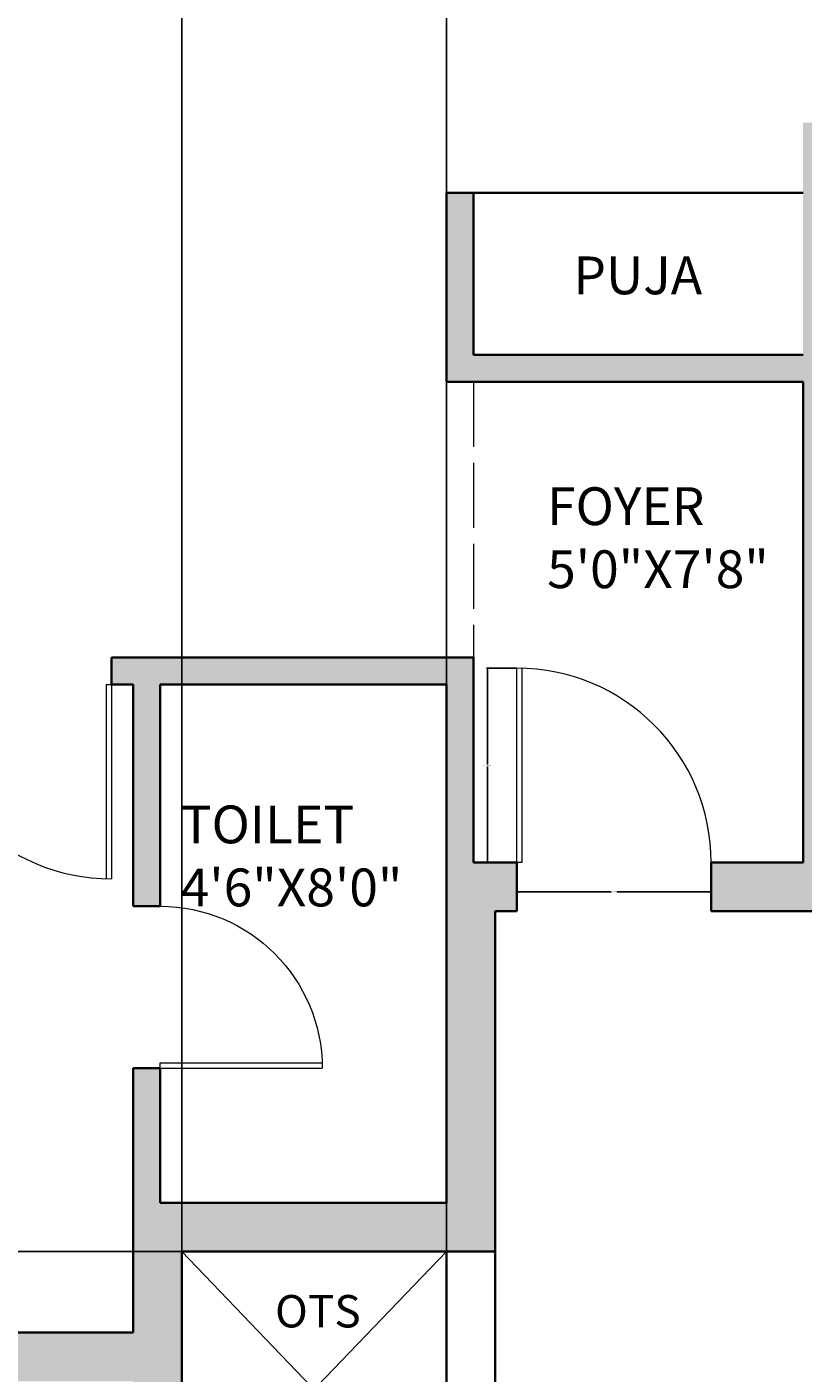
# Model space of a CAD drawing. Units: inches. Extents: x 2540 to 3167, y 3083 to 4007.
# Tile 11 of 15: x 2782 to 2926, y 3542 to 3791. Entities that reach past the tile are written whole.
import ezdxf

# ---------------------------------------------------------------- set-up
doc = ezdxf.new("R2010")
doc.units = ezdxf.units.IN
doc.linetypes.add('ACAD_ISO02W100', pattern=[15, 12, -3])
for name, color, linetype, lineweight in [('A-ANNO-DIMS', 2, 'Continuous', 18), ('A-AREA-IDEN', 7, 'Continuous', 18), ('A-DOOR', 4, 'Continuous', 18), ('A-FLOR-OPEN', 8, 'Continuous', 13)]:
    doc.layers.add(name, color=color, linetype=linetype, lineweight=lineweight)
for name, color, linetype, lineweight, true_color in [('A-WALL', 143, 'Continuous', 35, 0x7aafdf), ('A-WALL-OVHD', 143, 'ACAD_ISO02W100', 18, 0x7aafdf), ('A-WALL-PATT', 143, 'Continuous', 13, 0x7aafdf)]:
    doc.layers.add(name, color=color, linetype=linetype, lineweight=lineweight, true_color=true_color)
doc.styles.get("Standard").update_dxf_attribs({"font": 'arial.ttf'})
doc.dimstyles.get("Standard").update_dxf_attribs({"dimtxt": 0.18, "dimasz": 0.18, "dimexe": 0.18, "dimexo": 0.0625, "dimgap": 0.09, "dimtad": 0, "dimtih": 1, "dimtoh": 1, "dimdec": 4, "dimzin": 0, "dimdsep": 46, "dimtxsty": 'Standard', "dimcen": 0.09, "dimadec": 0, "dimazin": 0, "dimtfac": 1, "dimtdec": 4, "dimtofl": 0, "dimtmove": 0, "dimatfit": 3, "dimfxl": 1, "dimtolj": 1, "dimtzin": 0, "dimarcsym": 0})

# ---------------------------------------------------------------- blocks, each defined once
blk = doc.blocks.new('DOOR-SWING-36IN')
for p, q in [((36, 0), (0, 0)), ((36, 1), (0.01, 1)), ((36, 1), (36, 0))]:
    blk.add_line(p, q)
blk.add_arc((36, 0), 36, 90, 180)
blk = doc.blocks.new('DOOR-SWING-30IN')
for p, q in [((0, 0), (0, 30)), ((1, 0), (1, 29.98)), ((0, 0), (1, 0))]:
    blk.add_line(p, q)
blk.add_arc((0, 0), 30, 0, 90)
blk = doc.blocks.new('*D19')
at = {"layer": 'A-ANNO-DIMS', "color": 0, "lineweight": -2, "transparency": 16777216}
for p, q in [((2872.45, 3672.71), (2866.93, 3672.71)), ((2867.11, 3672.53), (2867.11, 3654.9)), ((2867.11, 3636.89), (2867.11, 3654.53)), ((2872.45, 3636.71), (2866.93, 3636.71))]:
    blk.add_line(p, q, dxfattribs=at)
at = {"layer": 'A-ANNO-DIMS', "color": 0, "transparency": 16777216}
for points in [[(2867.08, 3672.53), (2867.14, 3672.53), (2867.11, 3672.71)], [(2867.08, 3636.89), (2867.14, 3636.89), (2867.11, 3636.71)]]:
    blk.add_solid(points, dxfattribs=at)
at = {"layer": 'Defpoints', "color": 0, "transparency": 16777216}
for p in [(2872.51, 3672.71), (2867.11, 3636.71), (2872.51, 3636.71)]:
    blk.add_point(p, dxfattribs=at)
at = {"layer": 'A-ANNO-DIMS', "color": 0, "transparency": 16777216, "insert": (2867.11, 3654.71), "char_height": 0.18, "attachment_point": 5}
blk.add_mtext('\\A1;DOOR 36 TYP.', dxfattribs=at)
blk = doc.blocks.new('*D20')
at = {"layer": 'A-ANNO-DIMS', "color": 0, "lineweight": -2, "transparency": 16777216}
for p, q in [((2872.51, 3636.65), (2872.51, 3631.13)), ((2908.51, 3636.65), (2908.51, 3631.13)), ((2872.69, 3631.31), (2889.98, 3631.31)), ((2908.33, 3631.31), (2891.04, 3631.31))]:
    blk.add_line(p, q, dxfattribs=at)
at = {"layer": 'A-ANNO-DIMS', "color": 0, "transparency": 16777216}
for points in [[(2872.69, 3631.34), (2872.69, 3631.28), (2872.51, 3631.31)], [(2908.33, 3631.34), (2908.33, 3631.28), (2908.51, 3631.31)]]:
    blk.add_solid(points, dxfattribs=at)
at = {"layer": 'Defpoints', "color": 0, "transparency": 16777216}
for p in [(2872.51, 3636.71), (2908.51, 3636.71), (2908.51, 3631.31)]:
    blk.add_point(p, dxfattribs=at)
at = {"layer": 'A-ANNO-DIMS', "color": 0, "transparency": 16777216, "insert": (2890.51, 3631.31), "char_height": 0.18, "attachment_point": 5}
blk.add_mtext('\\A1;36 TYP.', dxfattribs=at)
blk = doc.blocks.new('*D44')
at = {"layer": 'A-ANNO-DIMS', "color": 0, "lineweight": -2, "transparency": 16777216}
for p, q in [((2771.45, 3964.71), (2540.23, 3964.71)), ((2540.41, 3964.53), (2540.41, 3545.4)), ((2540.41, 3125.89), (2540.41, 3545.03)), ((2810.45, 3125.71), (2540.23, 3125.71))]:
    blk.add_line(p, q, dxfattribs=at)
at = {"layer": 'A-ANNO-DIMS', "color": 0, "transparency": 16777216}
for points in [[(2540.38, 3964.53), (2540.44, 3964.53), (2540.41, 3964.71)], [(2540.38, 3125.89), (2540.44, 3125.89), (2540.41, 3125.71)]]:
    blk.add_solid(points, dxfattribs=at)
at = {"layer": 'Defpoints', "color": 0, "transparency": 16777216}
for p in [(2540.41, 3964.71), (2771.51, 3964.71), (2810.51, 3125.71)]:
    blk.add_point(p, dxfattribs=at)
at = {"layer": 'A-ANNO-DIMS', "color": 0, "transparency": 16777216, "insert": (2540.41, 3545.21), "char_height": 0.18, "attachment_point": 5}
blk.add_mtext('\\A1;839', dxfattribs=at)
blk = doc.blocks.new('*D55')
at = {"layer": 'A-ANNO-DIMS', "color": 0, "lineweight": -2, "transparency": 16777216}
for p, q in [((2868.51, 3564.65), (2868.51, 3083.43)), ((2930.51, 3543.65), (2930.51, 3083.43)), ((2868.69, 3083.61), (2899.29, 3083.61)), ((2930.33, 3083.61), (2899.73, 3083.61))]:
    blk.add_line(p, q, dxfattribs=at)
at = {"layer": 'A-ANNO-DIMS', "color": 0, "transparency": 16777216}
for points in [[(2868.69, 3083.64), (2868.69, 3083.58), (2868.51, 3083.61)], [(2930.33, 3083.64), (2930.33, 3083.58), (2930.51, 3083.61)]]:
    blk.add_solid(points, dxfattribs=at)
at = {"layer": 'Defpoints', "color": 0, "transparency": 16777216}
for p in [(2868.51, 3564.71), (2930.51, 3543.71), (2930.51, 3083.61)]:
    blk.add_point(p, dxfattribs=at)
at = {"layer": 'A-ANNO-DIMS', "color": 0, "transparency": 16777216, "insert": (2899.51, 3083.61), "char_height": 0.18, "attachment_point": 5}
blk.add_mtext('\\A1;62', dxfattribs=at)
blk = doc.blocks.new('*D56')
at = {"layer": 'A-ANNO-DIMS', "color": 0, "lineweight": -2, "transparency": 16777216}
for p, q in [((2810.51, 3564.78), (2810.51, 4006.99)), ((2810.69, 4006.81), (2834.79, 4006.81)), ((2859.33, 4006.81), (2835.23, 4006.81)), ((2859.51, 3564.78), (2859.51, 4006.99))]:
    blk.add_line(p, q, dxfattribs=at)
at = {"layer": 'A-ANNO-DIMS', "color": 0, "transparency": 16777216}
for points in [[(2810.69, 4006.84), (2810.69, 4006.78), (2810.51, 4006.81)], [(2859.33, 4006.84), (2859.33, 4006.78), (2859.51, 4006.81)]]:
    blk.add_solid(points, dxfattribs=at)
at = {"layer": 'Defpoints', "color": 0, "transparency": 16777216}
for p in [(2859.51, 4006.81), (2810.51, 3564.71), (2859.51, 3564.71)]:
    blk.add_point(p, dxfattribs=at)
at = {"layer": 'A-ANNO-DIMS', "color": 0, "transparency": 16777216, "insert": (2835.01, 4006.81), "char_height": 0.18, "attachment_point": 5}
blk.add_mtext('\\A1;49', dxfattribs=at)
blk = doc.blocks.new('*D57')
at = {"layer": 'A-ANNO-DIMS', "color": 0, "lineweight": -2, "transparency": 16777216}
for p, q in [((2810.45, 3564.71), (2540.23, 3564.71)), ((2540.41, 3564.53), (2540.41, 3539.4)), ((2540.41, 3513.89), (2540.41, 3539.03)), ((2810.45, 3513.71), (2540.23, 3513.71))]:
    blk.add_line(p, q, dxfattribs=at)
at = {"layer": 'A-ANNO-DIMS', "color": 0, "transparency": 16777216}
for points in [[(2540.38, 3564.53), (2540.44, 3564.53), (2540.41, 3564.71)], [(2540.38, 3513.89), (2540.44, 3513.89), (2540.41, 3513.71)]]:
    blk.add_solid(points, dxfattribs=at)
at = {"layer": 'Defpoints', "color": 0, "transparency": 16777216}
for p in [(2810.51, 3564.71), (2540.41, 3513.71), (2810.51, 3513.71)]:
    blk.add_point(p, dxfattribs=at)
at = {"layer": 'A-ANNO-DIMS', "color": 0, "transparency": 16777216, "insert": (2540.41, 3539.21), "char_height": 0.18, "attachment_point": 5}
blk.add_mtext('\\A1;51', dxfattribs=at)

msp = doc.modelspace()

# ---------------------------------------------------------------- hatches: boundary and pattern name
at = {"layer": 'A-WALL-PATT'}
h = msp.add_hatch(color=256, dxfattribs=at)
h.dxf.hatch_style = 1
h.paths.add_polyline_path([(2805.51, 3803.71), (2800.51, 3803.71), (2800.51, 3799.71), (2621.51, 3799.71), (2621.51, 3823.71), (2612.51, 3823.71), (2612.51, 3794.71), (2636.51, 3794.71), (2636.51, 3782.71), (2645.51, 3782.71), (2645.51, 3794.71), (2805.51, 3794.71)])
h.paths.add_polyline_path([(2810.51, 3564.71), (2868.51, 3564.71), (2868.51, 3627.71), (2872.51, 3627.71), (2872.51, 3636.71), (2864.51, 3636.71), (2864.51, 3674.71), (2797.51, 3674.71), (2797.51, 3669.71), (2801.51, 3669.71), (2801.51, 3628.63), (2806.51, 3628.63), (2806.51, 3669.71), (2859.51, 3669.71), (2859.51, 3573.71), (2806.51, 3573.71), (2806.51, 3598.63), (2801.51, 3598.63), (2801.51, 3549.71), (2645.51, 3549.71), (2645.51, 3573.71), (2636.51, 3573.71), (2636.51, 3516.71), (2645.51, 3516.71), (2645.51, 3540.71), (2801.51, 3540.71), (2801.51, 3504.71), (2801.51, 3500.71), (2806.51, 3500.71), (2806.51, 3504.71), (2859.51, 3504.71), (2859.51, 3420.71), (2806.51, 3420.71), (2806.51, 3470.71), (2801.51, 3470.71), (2801.51, 3420.71), (2797.51, 3420.71), (2797.51, 3415.71), (2864.51, 3415.71), (2864.51, 3453.71), (2868.51, 3453.71), (2868.51, 3513.71), (2810.51, 3513.71)])
h.paths.add_polyline_path([(2645.51, 3415.71), (2761.51, 3415.71), (2761.51, 3420.71), (2645.51, 3420.71), (2645.51, 3444.71), (2636.51, 3444.71), (2636.51, 3403.71), (2645.51, 3403.71)])
h.paths.add_polyline_path([(2645.51, 3307.71), (2636.51, 3307.71), (2636.51, 3295.71), (2612.51, 3295.71), (2612.51, 3149.71), (2645.51, 3149.71), (2645.51, 3158.71), (2621.51, 3158.71), (2621.51, 3290.71), (2801.51, 3290.71), (2801.51, 3286.71), (2806.51, 3286.71), (2806.51, 3295.71), (2645.51, 3295.71)])
h.paths.add_polyline_path([(2762.01, 3158.71), (2746.51, 3158.71), (2746.51, 3240.71), (2750.51, 3240.71), (2750.51, 3245.71), (2741.51, 3245.71), (2741.51, 3158.71), (2717.51, 3158.71), (2717.51, 3149.71), (2762.01, 3149.71)], flags=17)
h.paths.add_polyline_path([(2810.51, 3173.71), (2822.51, 3173.71), (2822.51, 3182.71), (2806.51, 3182.71), (2806.51, 3250.71), (2801.51, 3250.71), (2801.51, 3245.71), (2780.51, 3245.71), (2780.51, 3240.71), (2801.51, 3240.71), (2801.51, 3158.71), (2786.01, 3158.71), (2786.01, 3149.71), (2810.51, 3149.71)])
h.paths.add_polyline_path([(2931.51, 3290.71), (2935.51, 3290.71), (2935.51, 3295.71), (2926.51, 3295.71), (2926.51, 3182.71), (2910.51, 3182.71), (2910.51, 3173.71), (2922.51, 3173.71), (2922.51, 3149.71), (2987.51, 3149.71), (2987.51, 3158.71), (2931.51, 3158.71)])
h.paths.add_polyline_path([(3124.51, 3295.71), (3086.51, 3295.71), (3018.51, 3295.71), (3018.51, 3290.71), (3115.51, 3290.71), (3115.51, 3158.71), (3059.51, 3158.71), (3059.51, 3149.71), (3124.51, 3149.71)])
h.paths.add_polyline_path([(2988.51, 3295.71), (2984.51, 3295.71), (2984.51, 3349.71), (3086.51, 3349.71), (3086.51, 3320.71), (3124.51, 3320.71), (3124.51, 3354.71), (3071.51, 3354.71), (3071.51, 3358.71), (3062.51, 3358.71), (3062.51, 3354.71), (2979.51, 3354.71), (2979.51, 3295.71), (2971.51, 3295.71), (2971.51, 3290.71), (2988.51, 3290.71)])
h.paths.add_polyline_path([(3095.51, 3325.71), (3095.51, 3349.71), (3119.51, 3349.71), (3119.51, 3325.71)], flags=16)
h.paths.add_polyline_path([(3124.51, 3462.71), (3071.51, 3462.71), (3071.51, 3627.71), (3124.51, 3627.71), (3124.51, 3693.71), (3095.51, 3693.71), (3095.51, 3702.71), (3086.51, 3702.71), (3086.51, 3684.71), (3086.51, 3636.71), (2930.51, 3636.71), (2930.51, 3768.71), (2934.51, 3768.71), (2934.51, 3773.71), (2930.51, 3773.71), (2925.51, 3773.71), (2925.51, 3730.71), (2864.51, 3730.71), (2864.51, 3760.71), (2859.51, 3760.71), (2859.51, 3725.71), (2925.51, 3725.71), (2925.51, 3636.71), (2908.51, 3636.71), (2908.51, 3627.71), (3062.51, 3627.71), (3062.51, 3543.71), (2930.51, 3543.71), (2930.51, 3534.71), (2993.51, 3534.71), (2993.51, 3516.71), (3002.51, 3516.71), (3002.51, 3534.71), (3062.51, 3534.71), (3062.51, 3462.71), (3002.51, 3462.71), (3002.51, 3480.71), (2993.51, 3480.71), (2993.51, 3462.71), (2916.51, 3462.71), (2916.51, 3453.71), (2926.51, 3453.71), (2926.51, 3361.71), (2859.51, 3361.71), (2859.51, 3338.71), (2864.51, 3338.71), (2864.51, 3356.71), (2926.51, 3356.71), (2926.51, 3338.71), (2931.51, 3338.71), (2931.51, 3453.71), (3062.51, 3453.71), (3062.51, 3448.21), (3071.51, 3448.21), (3071.51, 3453.71), (3124.51, 3453.71)])

# ---------------------------------------------------------------- linework, layer by layer
at = {"layer": 'A-FLOR-OPEN'}
for p, q in [((2859.51, 3513.71), (2810.51, 3564.71)), ((2810.51, 3513.71), (2859.51, 3564.71))]:
    msp.add_line(p, q, dxfattribs=at)
at = {"layer": 'A-WALL'}
for p, q in [((2859.51, 3760.71), (2925.51, 3760.71)), ((2859.51, 3760.71), (2859.51, 3725.71)), ((2864.51, 3760.71), (2864.51, 3730.71)), ((2864.51, 3730.71), (2925.51, 3730.71)), ((2859.51, 3725.71), (2925.51, 3725.71)), ((2925.51, 3725.71), (2925.51, 3636.71)), ((2797.51, 3674.71), (2797.51, 3669.71)), ((2797.51, 3674.71), (2864.51, 3674.71)), ((2864.51, 3674.71), (2864.51, 3636.71)), ((2797.51, 3669.71), (2801.51, 3669.71)), ((2801.51, 3669.71), (2801.51, 3628.63)), ((2806.51, 3669.71), (2806.51, 3628.63)), ((2806.51, 3669.71), (2859.51, 3669.71)), ((2859.51, 3669.71), (2859.51, 3573.71)), ((2864.51, 3636.71), (2872.51, 3636.71)), ((2872.51, 3636.71), (2872.51, 3627.71)), ((2908.51, 3636.71), (2908.51, 3627.71)), ((2908.51, 3636.71), (2925.51, 3636.71)), ((2801.51, 3628.63), (2806.51, 3628.63)), ((2868.51, 3627.71), (2872.51, 3627.71)), ((2868.51, 3627.71), (2868.51, 3453.71)), ((2908.51, 3627.71), (3062.51, 3627.71)), ((2801.51, 3598.63), (2806.51, 3598.63)), ((2801.51, 3598.63), (2801.51, 3549.71)), ((2806.51, 3598.63), (2806.51, 3573.71)), ((2806.51, 3573.71), (2859.51, 3573.71)), ((2810.51, 3564.71), (2868.51, 3564.71)), ((2810.51, 3564.71), (2810.51, 3513.71)), ((2859.51, 3564.71), (2859.51, 3513.71)), ((2645.51, 3549.71), (2801.51, 3549.71))]:
    msp.add_line(p, q, dxfattribs=at)
at = {"layer": 'A-WALL-OVHD'}
for p, q in [((2859.51, 3725.71), (2859.51, 3674.71)), ((2864.51, 3725.71), (2864.51, 3674.71))]:
    msp.add_line(p, q, dxfattribs=at)

# ---------------------------------------------------------------- block references
at = {"layer": 'A-DOOR'}
for p, rotation in [((2872.51, 3672.71), 269.9999999999987), ((2797.51, 3633.71), 89.99999999999872)]:
    msp.add_blockref('DOOR-SWING-36IN', p, dxfattribs=dict(at, rotation=rotation))
at = {"layer": 'A-DOOR', "extrusion": (0, 0, -1), "zscale": -1, "rotation": 90.00000000000756}
msp.add_blockref('DOOR-SWING-30IN', (-2806.51, 3598.63), dxfattribs=at)

# ---------------------------------------------------------------- texts
at = {"layer": 'A-AREA-IDEN', "attachment_point": 1}
for s, width, insert, char_height in [('PUJA', 34.4573, (2882.99, 3748.92), 7), ('FOYER\\P5\'0"X7\'8"', 38.2617, (2878.14, 3706.19), 7), ('TOILET\\P4\'6"X8\'0"', 75.6369, (2810.31, 3647.28), 7), ('OTS', 23.7199, (2827.78, 3556.66), 6)]:
    msp.add_mtext_dynamic_manual_height_columns(s, width=width, gutter_width=12.5, heights=[0], dxfattribs=dict(at, insert=insert, char_height=char_height))

# ---------------------------------------------------------------- dimensions: what is measured, and where the dimension line sits
at = {"layer": 'A-ANNO-DIMS'}
for base, p1, p2, picture, middle in [((2859.51, 4006.81), (2810.51, 3564.71), (2859.51, 3564.71), '*D56', (2835.01, 4006.81)), ((2930.51, 3083.61), (2868.51, 3564.71), (2930.51, 3543.71), '*D55', (2899.51, 3083.61))]:
    dim = msp.add_linear_dim(base=base, p1=p1, p2=p2, dimstyle='Standard', override={"dimdec": 0, "dimlfac": 1, "dimrnd": 0, "dimzin": 0, "dimdsep": 46, "dimlunit": 2}, dxfattribs=at)
    dim.commit()
    dim.dimension.update_dxf_attribs({"geometry": picture, "text_midpoint": middle})
for base, p1, p2, picture, middle in [((2540.41, 3964.71), (2810.51, 3125.71), (2771.51, 3964.71), '*D44', (2540.41, 3545.21)), ((2540.41, 3513.71), (2810.51, 3564.71), (2810.51, 3513.71), '*D57', (2540.41, 3539.21))]:
    dim = msp.add_linear_dim(base=base, p1=p1, p2=p2, angle=90, dimstyle='Standard', override={"dimdec": 0, "dimlfac": 1, "dimrnd": 0, "dimzin": 0, "dimdsep": 46, "dimlunit": 2}, dxfattribs=at)
    dim.commit()
    dim.dimension.update_dxf_attribs({"geometry": picture, "text_midpoint": middle})
dim = msp.add_linear_dim(base=(2867.11, 3636.71), p1=(2872.51, 3672.71), p2=(2872.51, 3636.71), angle=270, text='DOOR <> TYP.', dimstyle='Standard', override={"dimdec": 0, "dimlfac": 1, "dimrnd": 0, "dimzin": 0, "dimdsep": 46, "dimlunit": 2}, dxfattribs=at)
dim.commit()
dim.dimension.update_dxf_attribs({"geometry": '*D19', "text_midpoint": (2867.11, 3654.71)})
dim = msp.add_linear_dim(base=(2908.51, 3631.31), p1=(2872.51, 3636.71), p2=(2908.51, 3636.71), text='<> TYP.', dimstyle='Standard', override={"dimdec": 0, "dimlfac": 1, "dimrnd": 0, "dimzin": 0, "dimdsep": 46, "dimlunit": 2}, dxfattribs=at)
dim.commit()
dim.dimension.update_dxf_attribs({"geometry": '*D20', "text_midpoint": (2890.51, 3631.31)})

doc.saveas('drawing.dxf')
